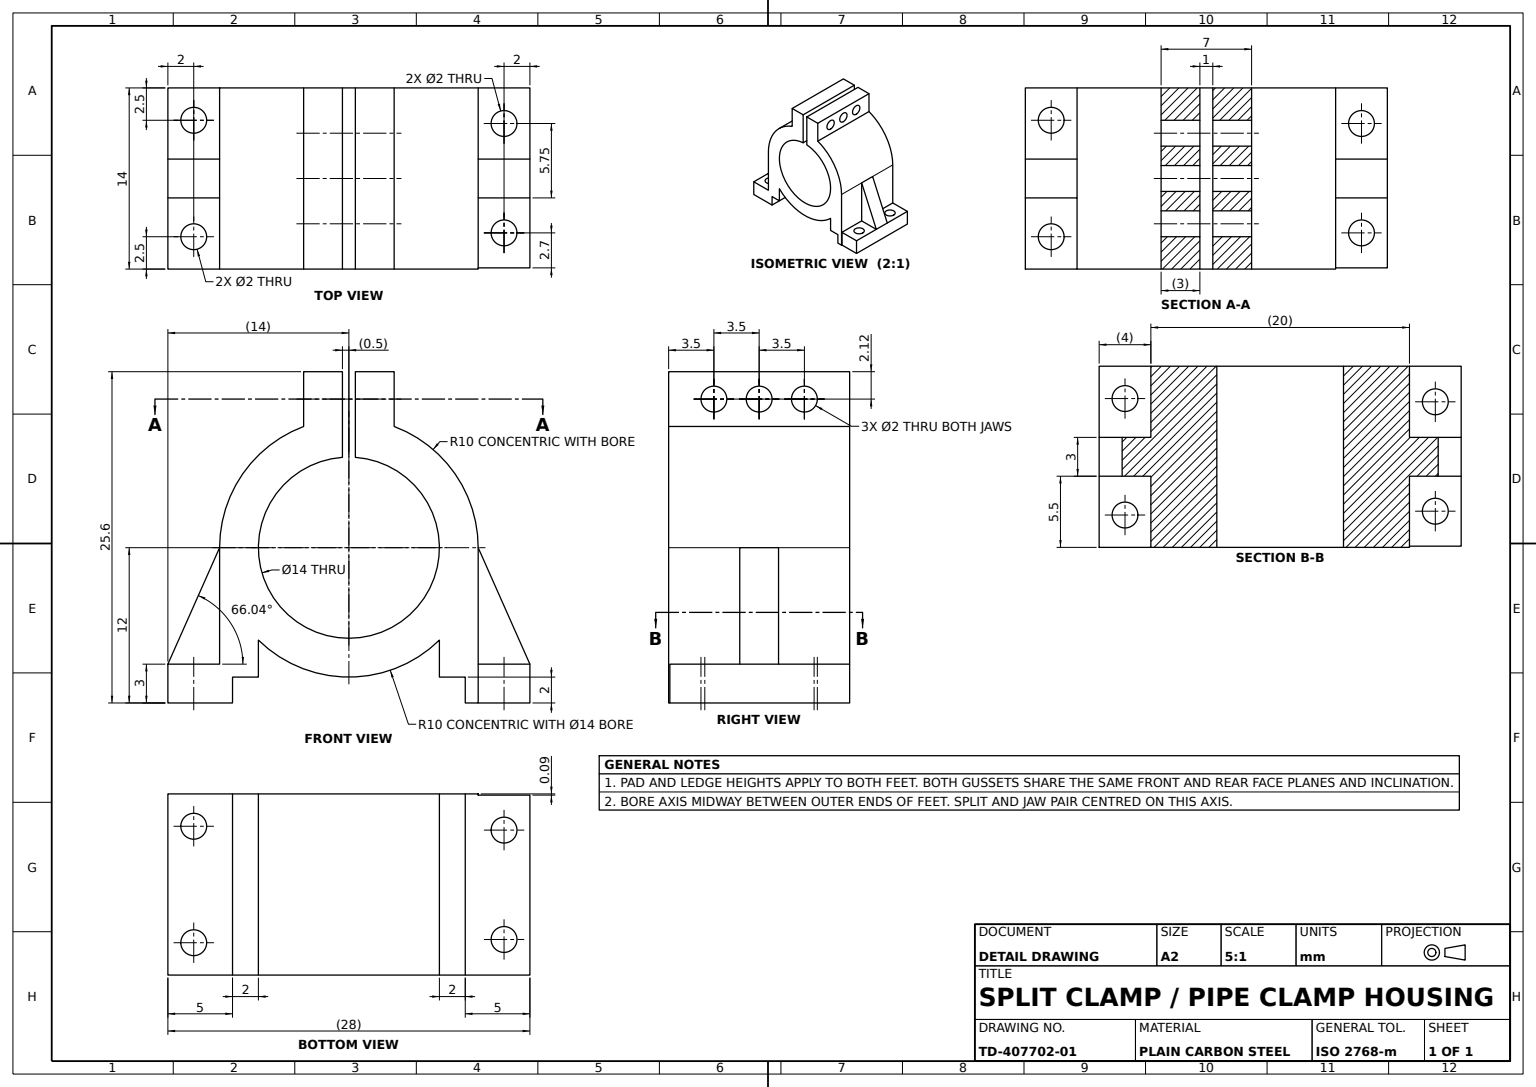
SolidWorks part; units mm, degrees
material "Plain Carbon Steel"
ref_plane "Front Plane" through (0, 0, 0) normal (0, 0, 1) x (1, 0, 0)
ref_plane "Top Plane" through (0, 0, 0) normal (0, 1, 0) x (1, 0, 0)
ref_plane "Right Plane" through (0, 0, 0) normal (1, 0, 0) x (0, 0, -1)
sketch "Base Block Sketch" plane through (0, 0, 0) normal (0, 1, 0) x (1, 0, 0)
  circle A0 centre (0, 0) radius 7
  circle A1 centre (0, 0) radius 10
  dimension "D1" = 14
  dimension "D2" = 20
extrude "Base Block" add sketch "Base Block Sketch" along normal blind 14
sketch "Clamp Ring Sketch" plane through (0, 14, 0) normal (0, 1, 0) x (1, 0, 0)
  line L0 (10, 0) -> (10, -12)
  line L1 (-10, 0) -> (-10, -12)
  line L2 (7, 0) -> (7, -12)
  line L3 (-7, 0) -> (-7, -12)
  line L4 (-10, -12) -> (-7, -12)
  line L5 (7, -12) -> (10, -12)
  circle A0 centre (0, 0) radius 10 construction
  arc A1 (-2.795, -9.6015) -> (9.563, 2.9237) centre (0, 0) ccw
  circle A2 centre (0, 0) radius 7 construction
  arc A3 (-7, 0) -> (7, 0) centre (0, 0) ccw
  arc A4 (-10, 0) -> (9.563, 2.9237) centre (0, 0) ccw
  circle M10 centre (0, 0) radius 10
  circle M11 centre (0, 0) radius 7
  dimension "D2" = 9.563
  dimension "D1" = 12
  dimension "D3" = 2.795
extrude "Clamp Ring" add sketch "Clamp Ring Sketch" against normal blind 14 contours L1 L4 L3 M10 | L3 L2 M11 M10 | L3 L2 M11 M10 | L2 L5 L0 M10
sketch "Side Rib Sketch" plane through (0, 0, 0) normal (1, 0, 0) x (0, 0, -1)
  line L1 (10, 14) -> (13.6, 14)
  line L2 (10, 14) -> (10, 0)
  line L3 (10, 0) -> (13.6, 0)
  line L4 (13.6, 14) -> (13.6, 0)
  dimension "D1" = 3.6
  dimension "D2" = 14
extrude "Side Rib" add sketch "Side Rib Sketch" along normal mid plane 7 separate body
sketch "Rib Infill Sketch" plane through (0, 14, 0) normal (0, 1, 0) x (1, 0, 0)
  line L0 (-3.5, 10) -> (-3.5, 9.3675)
  line L1 (3.5, 10) -> (3.5, 9.3675)
  line L7 (-3.5, 13.6) -> (-3.5, 10)
  line L8 (-3.5, 10) -> (3.5, 10)
  line L9 (3.5, 10) -> (3.5, 13.6)
  line L10 (3.5, 13.6) -> (-3.5, 13.6)
  line L12 (-3.5, 10) -> (3.5, 10)
  arc A0 (3.5, 9.3675) -> (-3.5, 9.3675) centre (0, 0) ccw
  arc M12 (10, 0) -> (-10, 0) centre (0, 0) ccw
  dimension "D1" = 0
extrude "Rib Infill" add sketch "Rib Infill Sketch" against normal blind 14 contours L12 L0 M12 | L12 L1 M12
sketch "Mounting Ear A Sketch" plane through (0, 0, 12) normal (0, 0, 1) x (1, 0, 0)
  line L1 (10, 0) -> (14, 0)
  line L2 (10, 0) -> (10, 13.9063)
  line L3 (10, 13.9063) -> (14, 13.9063)
  line L4 (14, 0) -> (14, 13.9063)
  line L5 (7, 14) -> (10, 14) construction
  dimension "D1" = 4
  dimension "D2" = 0.0937
extrude "Mounting Ear A" add sketch "Mounting Ear A Sketch" against normal blind 3
sketch "Mounting Ear B Sketch" plane through (0, 0, 12) normal (0, 0, 1) x (1, 0, 0)
  line L1 (-10, 14) -> (-14, 14)
  line L2 (-10, 14) -> (-10, 0)
  line L3 (-10, 0) -> (-14, 0)
  line L4 (-14, 14) -> (-14, 0)
  line L5 (-10, 14) -> (-7, 14) construction
  dimension "D1" = 4
  dimension "D2" = 14
extrude "Mounting Ear B" add sketch "Mounting Ear B Sketch" against normal blind 3
sketch "Clamp Slit A Sketch" plane through (0, 14, 0) normal (0, 1, 0) x (1, 0, 0)
  line L2 (-7, -12) -> (-9, -12)
  line L3 (-7, -12) -> (-7, -10)
  line L5 (-7, -10) -> (-9, -10)
  line L6 (-9, -12) -> (-9, -10)
  dimension "D1" = 2
  dimension "D2" = 2
extrude "Clamp Slit A" cut sketch "Clamp Slit A Sketch" against normal blind 56
sketch "Clamp Slit B Sketch" plane through (0, 14, 0) normal (0, 1, 0) x (1, 0, 0)
  line L0 (9, -12) -> (9, -10)
  line L1 (7, -12) -> (10, -12) construction
  line L2 (9, -10) -> (7, -10)
  line L3 (7, -7.1414) -> (7, -12) construction
  line L4 (7, -10) -> (7, -12)
  line L5 (7, -12) -> (9, -12)
  dimension "D1" = 2
  dimension "D2" = 2
extrude "Clamp Slit B" cut sketch "Clamp Slit B Sketch" against normal blind 92
sketch "Triangular Relief Sketch" plane through (3.5, 0, 0) normal (1, 0, 0) x (0, 0, -1)
  line L0 (13.6, 14) -> (9.3675, 14) construction
  line L1 (9.3675, 0) -> (9.3675, 14) construction
  circle A0 centre (11.4837, 7) radius 1
  circle A1 centre (11.4837, 3.5) radius 1
  circle A2 centre (11.4837, 10.5) radius 1
  dimension "D1" = 2
  dimension "D2" = 2
  dimension "D3" = 2
  dimension "D4" = 3.5
  dimension "D5" = 3.5
  dimension "D6" = 2.1163
  dimension "D7" = 7
extrude "Triangular Relief Cut" cut sketch "Triangular Relief Sketch" along normal blind 54 and the other way blind 33
sketch "Rib Groove Sketch" plane through (0, 0, -13.6) normal (0, 0, -1) x (-1, 0, 0)
  line L0 (0, 14) -> (0, 0)
  line L1 (-3.5, 14) -> (3.5, 14) construction
  line L2 (-0.5, 14) -> (-0.5, 0)
  line L3 (0.5, 14) -> (0.5, 0)
  line L4 (-0.5, 14) -> (0.5, 14)
  line L5 (-0.5, 0) -> (0.5, 0)
  line M3 (3.5, 14) -> (-3.5, 14)
  line M5 (-3.5, 0) -> (3.5, 0)
  dimension "D1" = 0.5
  dimension "D2" = 0.5
extrude "Rib Groove Cut" cut sketch "Rib Groove Sketch" against normal blind 14 contours L3 L0 M3 M5 | L2 L0 M3 M5
ref_plane "Plane1" through (0, 7, 0) normal (0, 1, 0) x (1, 0, 0)
sketch "Ear A Gusset Sketch" plane through (0, 7, 0) normal (0, 1, 0) x (1, 0, 0)
  line L0 (14, -9) -> (10, 0)
  line L1 (10, 0) -> (10, -9)
  line L2 (10, -9) -> (14, -9)
extrude "Ear A Gusset" add sketch "Ear A Gusset Sketch" against normal mid plane 3
sketch "Ear A Holes Sketch" plane through (0, 0, 9) normal (0, 0, -1) x (-1, 0, 0)
  line L1 (-10, 8.5) -> (-14, 8.5) construction
  circle A0 centre (-12, 11.2032) radius 1
  circle A1 centre (-12, 2.75) radius 1
  dimension "D1" = 2
  dimension "D2" = 2
  dimension "D3" = 2
  dimension "D4" = 2
  dimension "D5" = 2.7032
  dimension "D6" = 5.75
extrude "Ear A Holes 2xØ2" cut sketch "Ear A Holes Sketch" against normal mid plane 13
sketch "Ear B Gusset Sketch" plane through (0, 7, 0) normal (0, 1, 0) x (1, 0, 0)
  line L0 (-10, 0) -> (-14, -9)
  line L1 (-14, -9) -> (-10, -9)
  line L2 (-10, -9) -> (-10, 0)
extrude "Ear B Gusset" add sketch "Ear B Gusset Sketch" along normal mid plane 3
sketch "Ear B Holes Sketch" plane through (0, 0, 9) normal (0, 0, -1) x (-1, 0, 0)
  line L1 (14, 14) -> (14, 8.5) construction
  circle A0 centre (12, 2.5) radius 1
  circle A1 centre (12, 11.5) radius 1
  dimension "D1" = 2
  dimension "D2" = 2
  dimension "D3" = 2.5
  dimension "D4" = 2.5
  dimension "D5" = 2
  dimension "D6" = 2
extrude "Ear B Holes 2xØ2" cut sketch "Ear B Holes Sketch" against normal mid plane 20
